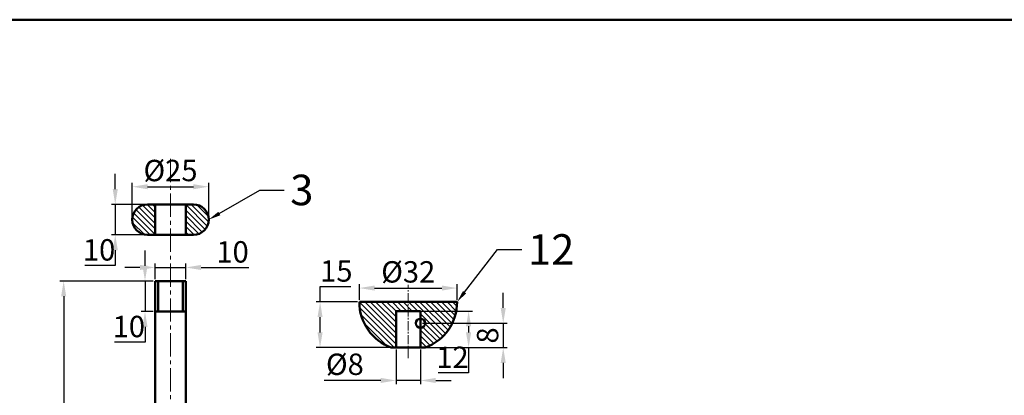
# Model space of a CAD drawing. Units: millimetres. Extents: x 434 to 1535, y -197 to 318.
# Tile 7 of 9: x 726 to 1049, y 195 to 318. Entities that reach past the tile are written whole.
import ezdxf
from ezdxf import colors
from ezdxf.entities.mleader import LeaderData, LeaderLine
from ezdxf.math import Vec2, Vec3

# ---------------------------------------------------------------- set-up
doc = ezdxf.new("R2010")
doc.units = ezdxf.units.MM
doc.header["$LTSCALE"] = 0.4
doc.linetypes.add('CENTER2', pattern=[28.575, 19.05, -3.175, 3.175, -3.175])
for name, color, linetype, lineweight in [('M-CNTR', 1, 'CENTER2', 18), ('M-DIMS', 2, 'Continuous', 25), ('M-HATC', 8, 'Continuous', 18), ('M-OUTL', 7, 'Continuous', 50), ('M-TEXT', 3, 'Continuous', 25)]:
    doc.layers.add(name, color=color, linetype=linetype, lineweight=lineweight)
doc.styles.get("Standard").update_dxf_attribs({"font": 'arial.ttf'})
doc.dimstyles.new('ISO-25', dxfattribs={"dimtxt": 7, "dimasz": 5, "dimexe": 1.25, "dimexo": 0.625, "dimtad": 1, "dimtoh": 1, "dimdec": 0, "dimtxsty": 'Standard', "dimcen": 2.5, "dimadec": 0, "dimazin": 0, "dimtfac": 1, "dimtdec": 0, "dimtmove": 0, "dimatfit": 3, "dimfxl": 1, "dimarcsym": 0})

# ---------------------------------------------------------------- blocks, each defined once
blk = doc.blocks.new('*U48')
at = {"layer": 'M-CNTR', "color": 0, "transparency": 16777216}
blk.add_line((0, 223.89), (0, -74.65), dxfattribs=at)
blk = doc.blocks.new('*D49')
at = {"layer": 'Defpoints', "color": 0, "ltscale": 0.4, "transparency": 16777216}
for p in [(770.74, 257.97), (757.65, 247.97), (770.74, 247.97)]:
    blk.add_point(p, dxfattribs=at)
at = {"layer": 'M-DIMS', "color": 0, "lineweight": -2, "ltscale": 0.4, "transparency": 16777216}
for p, q in [((757.65, 262.97), (757.65, 267.97)), ((770.11, 257.97), (756.4, 257.97)), ((757.65, 257.97), (757.65, 247.97)), ((770.11, 247.97), (756.4, 247.97)), ((757.65, 242.97), (757.65, 237.97)), ((757.65, 237.97), (747.68, 237.97))]:
    blk.add_line(p, q, dxfattribs=at)
at = {"layer": 'M-DIMS', "color": 0, "ltscale": 0.4, "transparency": 16777216}
for points in [[(756.82, 262.97), (758.49, 262.97), (757.65, 257.97)], [(756.82, 242.97), (758.49, 242.97), (757.65, 247.97)]]:
    blk.add_solid(points, dxfattribs=at)
at = {"layer": 'M-DIMS', "color": 0, "ltscale": 0.4, "transparency": 16777216, "insert": (752.36, 242.17), "char_height": 7, "attachment_point": 5}
blk.add_mtext('10', dxfattribs=at)
blk = doc.blocks.new('*D50')
at = {"layer": 'Defpoints', "color": 0, "ltscale": 0.4, "transparency": 16777216}
for p in [(788.24, 263.75), (763.24, 252.97), (788.24, 252.97)]:
    blk.add_point(p, dxfattribs=at)
at = {"layer": 'M-DIMS', "color": 0, "lineweight": -2, "ltscale": 0.4, "transparency": 16777216}
for p, q in [((763.24, 253.59), (763.24, 265)), ((788.24, 253.59), (788.24, 265)), ((768.24, 263.75), (783.24, 263.75))]:
    blk.add_line(p, q, dxfattribs=at)
at = {"layer": 'M-DIMS', "color": 0, "ltscale": 0.4, "transparency": 16777216}
for points in [[(768.24, 264.59), (768.24, 262.92), (763.24, 263.75)], [(783.24, 264.59), (783.24, 262.92), (788.24, 263.75)]]:
    blk.add_solid(points, dxfattribs=at)
at = {"layer": 'M-DIMS', "color": 0, "ltscale": 0.4, "transparency": 16777216, "insert": (775.74, 268.15), "char_height": 7, "attachment_point": 5}
blk.add_mtext('%%C25', dxfattribs=at)
blk = doc.blocks.new('*D51')
at = {"layer": 'Defpoints', "color": 0, "ltscale": 0.4, "transparency": 16777216}
for p in [(780.74, 237.31), (770.74, 232.87), (780.74, 232.87)]:
    blk.add_point(p, dxfattribs=at)
at = {"layer": 'M-DIMS', "color": 0, "lineweight": -2, "ltscale": 0.4, "transparency": 16777216}
for p, q in [((770.74, 233.5), (770.74, 238.56)), ((780.74, 233.5), (780.74, 238.56)), ((765.74, 237.31), (760.74, 237.31)), ((770.74, 237.31), (780.74, 237.31)), ((785.74, 237.31), (801.33, 237.31))]:
    blk.add_line(p, q, dxfattribs=at)
at = {"layer": 'M-DIMS', "color": 0, "ltscale": 0.4, "transparency": 16777216}
for points in [[(765.74, 238.15), (765.74, 236.48), (770.74, 237.31)], [(785.74, 238.15), (785.74, 236.48), (780.74, 237.31)]]:
    blk.add_solid(points, dxfattribs=at)
at = {"layer": 'M-DIMS', "color": 0, "ltscale": 0.4, "transparency": 16777216, "insert": (796.04, 241.51), "char_height": 7, "attachment_point": 5}
blk.add_mtext('10', dxfattribs=at)
blk = doc.blocks.new('*D52')
at = {"layer": 'Defpoints', "color": 0, "ltscale": 0.4, "transparency": 16777216}
for p in [(770.74, 232.87), (767.39, 222.87), (770.74, 222.87)]:
    blk.add_point(p, dxfattribs=at)
at = {"layer": 'M-DIMS', "color": 0, "lineweight": -2, "ltscale": 0.4, "transparency": 16777216}
for p, q in [((767.39, 237.87), (767.39, 242.87)), ((770.11, 232.87), (766.14, 232.87)), ((767.39, 232.87), (767.39, 222.87)), ((770.11, 222.87), (766.14, 222.87)), ((767.39, 217.87), (767.39, 212.87)), ((767.39, 212.87), (757.42, 212.87))]:
    blk.add_line(p, q, dxfattribs=at)
at = {"layer": 'M-DIMS', "color": 0, "ltscale": 0.4, "transparency": 16777216}
for points in [[(766.55, 237.87), (768.22, 237.87), (767.39, 232.87)], [(766.55, 217.87), (768.22, 217.87), (767.39, 222.87)]]:
    blk.add_solid(points, dxfattribs=at)
at = {"layer": 'M-DIMS', "color": 0, "ltscale": 0.4, "transparency": 16777216, "insert": (762.09, 217.07), "char_height": 7, "attachment_point": 5}
blk.add_mtext('10', dxfattribs=at)
blk = doc.blocks.new('*D53')
at = {"layer": 'Defpoints', "color": 0, "ltscale": 0.4, "transparency": 16777216}
for p in [(770.74, 232.87), (740.77, -32.13), (770.74, -32.13)]:
    blk.add_point(p, dxfattribs=at)
at = {"layer": 'M-DIMS', "color": 0, "lineweight": -2, "ltscale": 0.4, "transparency": 16777216}
for p, q in [((770.11, 232.87), (739.52, 232.87)), ((740.77, 227.87), (740.77, -27.13)), ((770.11, -32.13), (739.52, -32.13))]:
    blk.add_line(p, q, dxfattribs=at)
at = {"layer": 'M-DIMS', "color": 0, "ltscale": 0.4, "transparency": 16777216}
for points in [[(739.94, 227.87), (741.61, 227.87), (740.77, 232.87)], [(739.94, -27.13), (741.61, -27.13), (740.77, -32.13)]]:
    blk.add_solid(points, dxfattribs=at)
at = {"layer": 'M-DIMS', "color": 0, "ltscale": 0.4, "transparency": 16777216, "insert": (736.57, 100.37), "char_height": 7, "attachment_point": 5, "rotation": 90}
blk.add_mtext('265', dxfattribs=at)
blk = doc.blocks.new('*D95')
at = {"layer": 'Defpoints', "color": 0, "ltscale": 0.4, "transparency": 16777216}
for p in [(869.54, 230.57), (837.54, 226.05), (869.54, 226.05)]:
    blk.add_point(p, dxfattribs=at)
at = {"layer": 'M-DIMS', "color": 0, "lineweight": -2, "ltscale": 0.4, "transparency": 16777216}
for p, q in [((837.54, 226.68), (837.54, 231.82)), ((842.54, 230.57), (864.54, 230.57)), ((869.54, 226.68), (869.54, 231.82))]:
    blk.add_line(p, q, dxfattribs=at)
at = {"layer": 'M-DIMS', "color": 0, "ltscale": 0.4, "transparency": 16777216}
for points in [[(842.54, 231.4), (842.54, 229.74), (837.54, 230.57)], [(864.54, 231.4), (864.54, 229.74), (869.54, 230.57)]]:
    blk.add_solid(points, dxfattribs=at)
at = {"layer": 'M-DIMS', "color": 0, "ltscale": 0.4, "transparency": 16777216, "insert": (853.54, 234.96), "char_height": 7, "attachment_point": 5}
blk.add_mtext('%%C32', dxfattribs=at)
blk = doc.blocks.new('*D96')
at = {"layer": 'Defpoints', "color": 0, "ltscale": 0.4, "transparency": 16777216}
for p in [(837.54, 226.05), (824.68, 211.05), (847.97, 211.05)]:
    blk.add_point(p, dxfattribs=at)
at = {"layer": 'M-DIMS', "color": 0, "lineweight": -2, "ltscale": 0.4, "transparency": 16777216}
for p, q in [((824.68, 226.05), (824.68, 231.05)), ((824.68, 231.05), (834.72, 231.05)), ((836.91, 226.05), (823.43, 226.05)), ((824.68, 216.05), (824.68, 221.05)), ((847.34, 211.05), (823.43, 211.05))]:
    blk.add_line(p, q, dxfattribs=at)
at = {"layer": 'M-DIMS', "color": 0, "ltscale": 0.4, "transparency": 16777216}
for points in [[(823.85, 221.05), (825.51, 221.05), (824.68, 226.05)], [(823.85, 216.05), (825.51, 216.05), (824.68, 211.05)]]:
    blk.add_solid(points, dxfattribs=at)
at = {"layer": 'M-DIMS', "color": 0, "ltscale": 0.4, "transparency": 16777216, "insert": (830.01, 235.25), "char_height": 7, "attachment_point": 5}
blk.add_mtext('15', dxfattribs=at)
blk = doc.blocks.new('*D97')
at = {"layer": 'Defpoints', "color": 0, "ltscale": 0.4, "transparency": 16777216}
for p in [(849.54, 223.05), (849.54, 211.05), (873.29, 211.05)]:
    blk.add_point(p, dxfattribs=at)
at = {"layer": 'M-DIMS', "color": 0, "lineweight": -2, "ltscale": 0.4, "transparency": 16777216}
for p, q in [((850.16, 223.05), (874.54, 223.05)), ((873.29, 218.05), (873.29, 216.05)), ((850.16, 211.05), (874.54, 211.05)), ((873.29, 211.05), (873.29, 202.84)), ((873.29, 202.84), (863.36, 202.84))]:
    blk.add_line(p, q, dxfattribs=at)
at = {"layer": 'M-DIMS', "color": 0, "ltscale": 0.4, "transparency": 16777216}
for points in [[(872.45, 218.05), (874.12, 218.05), (873.29, 223.05)], [(872.45, 216.05), (874.12, 216.05), (873.29, 211.05)]]:
    blk.add_solid(points, dxfattribs=at)
at = {"layer": 'M-DIMS', "color": 0, "ltscale": 0.4, "transparency": 16777216, "insert": (868.01, 206.98), "char_height": 7, "attachment_point": 5}
blk.add_mtext('12', dxfattribs=at)
blk = doc.blocks.new('*D98')
at = {"layer": 'Defpoints', "color": 0, "ltscale": 0.4, "transparency": 16777216}
for p in [(857.54, 219.05), (857.54, 211.05), (884.62, 211.05)]:
    blk.add_point(p, dxfattribs=at)
at = {"layer": 'M-DIMS', "color": 0, "lineweight": -2, "ltscale": 0.4, "transparency": 16777216}
for p, q in [((884.62, 224.05), (884.62, 229.05)), ((858.16, 219.05), (885.87, 219.05)), ((884.62, 219.05), (884.62, 211.05)), ((858.16, 211.05), (885.87, 211.05)), ((884.62, 206.05), (884.62, 201.05))]:
    blk.add_line(p, q, dxfattribs=at)
at = {"layer": 'M-DIMS', "color": 0, "ltscale": 0.4, "transparency": 16777216}
for points in [[(883.79, 224.05), (885.46, 224.05), (884.62, 219.05)], [(883.79, 206.05), (885.46, 206.05), (884.62, 211.05)]]:
    blk.add_solid(points, dxfattribs=at)
at = {"layer": 'M-DIMS', "color": 0, "ltscale": 0.4, "transparency": 16777216, "insert": (880.42, 215.05), "char_height": 7, "attachment_point": 5, "rotation": 90}
blk.add_mtext('8', dxfattribs=at)
blk = doc.blocks.new('*D99')
at = {"layer": 'Defpoints', "color": 0, "ltscale": 0.4, "transparency": 16777216}
for p in [(849.54, 211.05), (857.54, 211.05), (857.54, 200.31)]:
    blk.add_point(p, dxfattribs=at)
at = {"layer": 'M-DIMS', "color": 0, "lineweight": -2, "ltscale": 0.4, "transparency": 16777216}
for p, q in [((849.54, 210.43), (849.54, 199.06)), ((857.54, 210.43), (857.54, 199.06)), ((844.54, 200.31), (826.07, 200.31)), ((857.54, 200.31), (849.54, 200.31)), ((862.54, 200.31), (867.54, 200.31))]:
    blk.add_line(p, q, dxfattribs=at)
at = {"layer": 'M-DIMS', "color": 0, "ltscale": 0.4, "transparency": 16777216}
for points in [[(844.54, 201.14), (844.54, 199.48), (849.54, 200.31)], [(862.54, 201.14), (862.54, 199.48), (857.54, 200.31)]]:
    blk.add_solid(points, dxfattribs=at)
at = {"layer": 'M-DIMS', "color": 0, "ltscale": 0.4, "transparency": 16777216, "insert": (832.8, 204.7), "char_height": 7, "attachment_point": 5}
blk.add_mtext('%%C8', dxfattribs=at)
blk = doc.blocks.new('DIE')
at = {"ltscale": 0.4}
for p, q in [((0, 15), (32, 15)), ((21.57, 0), (10.43, 0))]:
    blk.add_line(p, q, dxfattribs=at)
for start, end in [(180, 249.6359), (290.3641, 0)]:
    blk.add_arc((16, 15), 16, start, end, dxfattribs=at)

msp = doc.modelspace()

# ---------------------------------------------------------------- hatches: boundary and pattern name
at = {"layer": 'M-HATC', "ltscale": 0.4}
h = msp.add_hatch(dxfattribs=at)
h.set_pattern_fill('ANSI31', color=256, scale=0.4, angle=90)
h.set_pattern_definition([(135, (-18.9852, -70.3126), (-0.8980256, -0.8980256), [])])
h.paths.add_polyline_path([(768.24, 247.97), (770.74, 247.97), (770.74, 257.97), (768.24, 257.97, 1)])
h.paths.add_polyline_path([(780.74, 247.97), (783.24, 247.97, 1), (783.24, 257.97), (780.74, 257.97)])
h = msp.add_hatch(dxfattribs=at)
h.set_pattern_fill('ANSI31', color=256, scale=0.4, angle=90)
h.set_pattern_definition([(135, (287.3198, 336.1819), (-0.8980256, -0.8980256), [])])
h.paths.add_polyline_path([(849.54, 223.05), (853.54, 223.05), (853.54, 226.05), (837.54, 226.05, 0.313553), (847.97, 211.05), (849.54, 211.05)])
h.paths.add_polyline_path([(869.54, 226.05), (853.54, 226.05), (853.54, 223.05), (857.54, 223.05), (857.54, 220.55, -0.414214), (859.04, 219.05, -0.414214), (857.54, 217.55), (857.54, 211.05), (859.1, 211.05, 0.313553)])

# ---------------------------------------------------------------- linework, layer by layer
at = {"layer": 'M-CNTR', "ltscale": 0.4}
msp.add_line((853.54, 207.57), (853.54, 231.65), dxfattribs=at)
at = {"layer": 'M-OUTL', "ltscale": 0.4}
for p, q in [((770.74, 257.97), (770.74, 247.97)), ((780.74, 257.97), (780.74, 247.97)), ((770.74, 232.87), (770.74, 164.55)), ((770.74, 232.87), (780.74, 232.87)), ((771.74, 232.87), (771.74, 222.87)), ((779.74, 232.87), (779.74, 222.87)), ((780.74, 232.87), (780.74, 164.55)), ((770.74, 222.87), (780.74, 222.87)), ((849.54, 211.05), (849.54, 223.05)), ((857.54, 223.05), (849.54, 223.05)), ((857.54, 211.05), (857.54, 223.05))]:
    msp.add_line(p, q, dxfattribs=at)
msp.add_lwpolyline([(434.2, 318.45), (1535.47, 318.45), (1535.47, -197.48), (434.2, -197.48)], close=True, dxfattribs=at)
msp.add_lwpolyline([(768.24, 257.97, 1), (768.24, 247.97), (783.24, 247.97, 1), (783.24, 257.97)], format="xyb", close=True, dxfattribs=at)
msp.add_circle((857.54, 219.05), 1.5, dxfattribs=at)

# ---------------------------------------------------------------- block references
at = {"layer": 'M-CNTR'}
msp.add_blockref('*U48', (775.74, 49.02), dxfattribs=at)
at = {"layer": 'M-OUTL'}
msp.add_blockref('DIE', (837.54, 211.05), dxfattribs=at)

# ---------------------------------------------------------------- dimensions: what is measured, and where the dimension line sits
at = {"layer": 'M-DIMS', "ltscale": 0.4}
for base, p1, p2, picture, middle in [((788.24, 263.75), (763.24, 252.97), (788.24, 252.97), '*D50', (775.74, 268.15)), ((869.54, 230.57), (837.54, 226.05), (869.54, 226.05), '*D95', (853.54, 234.96))]:
    dim = msp.add_linear_dim(base=base, p1=p1, p2=p2, text='%%C<>', dimstyle='ISO-25', override={"dimclrd": 0, "dimclre": 0, "dimclrt": 0}, dxfattribs=at)
    dim.commit()
    dim.dimension.update_dxf_attribs({"geometry": picture, "text_midpoint": middle})
for base, p1, p2, picture, middle in [((757.65, 247.97), (770.74, 257.97), (770.74, 247.97), '*D49', (752.36, 242.17)), ((767.39, 222.87), (770.74, 232.87), (770.74, 222.87), '*D52', (762.09, 217.07)), ((740.77, -32.13), (770.74, 232.87), (770.74, -32.13), '*D53', (736.57, 100.37)), ((884.62, 211.05), (857.54, 219.05), (857.54, 211.05), '*D98', (880.42, 215.05))]:
    dim = msp.add_linear_dim(base=base, p1=p1, p2=p2, angle=90, dimstyle='ISO-25', override={"dimclrd": 0, "dimclre": 0, "dimclrt": 0}, dxfattribs=at)
    dim.commit()
    dim.dimension.update_dxf_attribs({"geometry": picture, "text_midpoint": middle})
dim = msp.add_linear_dim(base=(780.74, 237.31), p1=(770.74, 232.87), p2=(780.74, 232.87), dimstyle='ISO-25', override={"dimclrd": 0, "dimclre": 0, "dimclrt": 0}, dxfattribs=at)
dim.commit()
dim.dimension.update_dxf_attribs({"geometry": '*D51', "text_midpoint": (796.04, 241.51)})
for base, p1, p2, picture, middle in [((824.68, 211.05), (837.54, 226.05), (847.97, 211.05), '*D96', (830.01, 231.05)), ((873.29, 211.05), (849.54, 223.05), (849.54, 211.05), '*D97', (868.01, 202.84))]:
    dim = msp.add_linear_dim(base=base, p1=p1, p2=p2, angle=90, dimstyle='ISO-25', override={"dimclrd": 0, "dimclre": 0, "dimclrt": 0}, dxfattribs=at)
    dim.commit()
    dim.dimension.update_dxf_attribs({"geometry": picture, "text_midpoint": middle, "dimtype": 160})
dim = msp.add_linear_dim(base=(857.54, 200.31), p1=(849.54, 211.05), p2=(857.54, 211.05), text='%%C<>', dimstyle='ISO-25', override={"dimclrd": 0, "dimclre": 0, "dimclrt": 0}, dxfattribs=at)
dim.commit()
dim.dimension.update_dxf_attribs({"geometry": '*D99', "text_midpoint": (832.8, 200.31), "dimtype": 160})

# ---------------------------------------------------------------- leaders
at = {"layer": 'M-TEXT', "ltscale": 0.4}
ml = msp.add_multileader_mtext('Standard', dxfattribs=at)
ml.set_content('3', color=256)
ml.set_leader_properties()
ml.build(insert=Vec2(0, 0))
ctx = ml.context
ctx.base_point, ctx.char_height, ctx.plane_origin = Vec3(812.92, 262.6), 10, Vec3(788.24, 252.97)
notes = []
notes.append((ctx, [(0, (1, 1, 0), (804.92, 262.6), (1, 0), 8, [(0, [(788.24, 252.97)], 0, [])])]))
ctx.mtext.insert, ctx.mtext.flow_direction = Vec3(814.92, 267.69), 5
ml = msp.add_multileader_mtext('Standard', dxfattribs=at)
ml.set_content('12', color=256)
ml.set_leader_properties()
ml.build(insert=Vec2(0, 0))
ctx = ml.context
ctx.base_point, ctx.char_height, ctx.plane_origin = Vec3(890.75, 243.2), 10, Vec3(869.54, 226.05)
notes.append((ctx, [(0, (1, 1, 0), (882.75, 243.2), (1, 0), 8, [(0, [(869.54, 226.05)], 0, [])])]))
ctx.mtext.insert, ctx.mtext.flow_direction = Vec3(892.75, 248.2), 5
for ctx, leaders in notes:
    for number, flags, end, landing, length, lines in leaders:
        leader = LeaderData()
        leader.index, (leader.has_last_leader_line, leader.has_dogleg_vector, leader.attachment_direction) = number, flags
        leader.last_leader_point, leader.dogleg_vector, leader.dogleg_length = Vec3(end), Vec3(landing), length
        for number, points, colour, breaks in lines:
            line = LeaderLine()
            line.index, line.vertices, line.color, line.breaks = number, Vec3.list(points), colors.encode_raw_color(colour), breaks
            leader.lines.append(line)
        ctx.leaders.append(leader)

doc.saveas('drawing.dxf')
